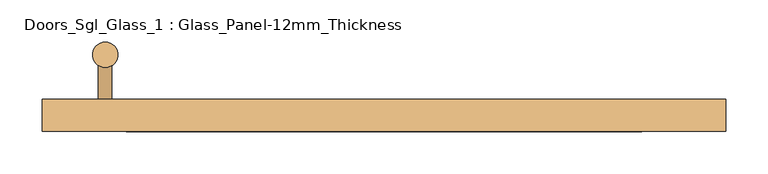
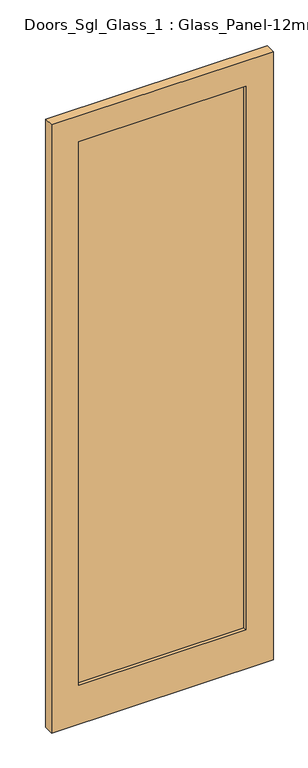
"""IFC4 building model written with IfcOpenShell, lengths in millimetres: door geometry, Doors_Sgl_Glass_1 : Glass_Panel-12mm_Thickness."""

from ifc_helpers import new_model, si_unit, point, frame, frame_2d, origin, place, context, project, spatial, polyline, circle_curve, trimmed, segment, composite_curve, outline, extrude, source, transform, mapped, element, save


def doors_sgl_glass_1_glass_panel_12mm_thickness_d76e1df9(model_context):
    return source(origin(), model_context, "Body", "SweptSolid", [
        extrude(outline(polyline([(306.4578978, 50.0), (306.4578978, 38.0), (-306.4578978, 38.0), (-306.4578978, 50.0), (306.4578978, 50.0)])), frame((0.0, 0.0, 150.0), z_axis=(0.0, 0.0, 1.0), x_axis=(1.0, 0.0, 0.0)), (0.0, 0.0, 1.0), 2105.0),
        extrude(outline(polyline([(0.0, -406.4578978), (0.0, 406.4578978), (2355.0, 406.4578978), (2355.0, -406.4578978), (0.0, -406.4578978)]), holes=[polyline([(2255.0, 306.4578978), (150.0, 306.4578978), (150.0, -306.4578978), (2255.0, -306.4578978), (2255.0, 306.4578978)])]), frame((0.0, 25.0, 0.0), z_axis=(0.0, 1.0, 0.0), x_axis=(0.0, 0.0, 1.0)), (0.0, 0.0, 1.0), 38.0),
        extrude(outline(composite_curve([segment(trimmed(circle_curve(frame_2d((1450.0, -331.4578978)), 8.0), [point((1450.0, -323.4578978))], [point((1450.0, -339.4578978))], False, "CARTESIAN"), True, "CONTINUOUS"), segment(trimmed(circle_curve(frame_2d((1450.0, -331.4578978)), 8.0), [point((1450.0, -339.4578978))], [point((1450.0, -323.4578978))], False, "CARTESIAN"), True, "CONTINUOUS")], self_intersect=False)), frame((0.0, 63.0, 0.0), z_axis=(0.0, 1.0, 0.0), x_axis=(0.0, 0.0, 1.0)), (0.0, 0.0, 1.0), 53.0),
        extrude(outline(composite_curve([segment(trimmed(circle_curve(frame_2d((750.0, -331.4578978)), 8.0), [point((750.0, -323.4578978))], [point((750.0, -339.4578978))], False, "CARTESIAN"), True, "CONTINUOUS"), segment(trimmed(circle_curve(frame_2d((750.0, -331.4578978)), 8.0), [point((750.0, -339.4578978))], [point((750.0, -323.4578978))], False, "CARTESIAN"), True, "CONTINUOUS")], self_intersect=False)), frame((0.0, 63.0, 0.0), z_axis=(0.0, 1.0, 0.0), x_axis=(0.0, 0.0, 1.0)), (0.0, 0.0, 1.0), 53.0),
        extrude(outline(composite_curve([segment(trimmed(circle_curve(frame_2d((-331.4578978, 116.0)), 15.0), [point((-331.4578978, 101.0))], [point((-331.4578978, 131.0))], False, "CARTESIAN"), True, "CONTINUOUS"), segment(trimmed(circle_curve(frame_2d((-331.4578978, 116.0)), 15.0), [point((-331.4578978, 131.0))], [point((-331.4578978, 101.0))], False, "CARTESIAN"), True, "CONTINUOUS")], self_intersect=False)), frame((0.0, 0.0, 650.0), z_axis=(0.0, 0.0, 1.0), x_axis=(1.0, 0.0, 0.0)), (0.0, 0.0, 1.0), 900.0),
    ])


if __name__ == "__main__":
    model = new_model("IFC4")
    model_context = context("Model", 3, world=origin())
    ifc_project = project(units=[si_unit("LENGTHUNIT", "METRE", prefix="MILLI")], contexts=[model_context])
    site = spatial("IfcSite", under=ifc_project)
    building = spatial("IfcBuilding", under=site)
    placement = place(None, origin())
    doors_sgl_glass_1_glass_panel_12mm_thickness_shape = doors_sgl_glass_1_glass_panel_12mm_thickness_d76e1df9(model_context)
    element("IfcDoor", 1, ObjectType="Doors_Sgl_Glass_1 : Glass_Panel-12mm_Thickness", at=placement, inside=building, context=model_context, shape_type="MappedRepresentation", body=[
        mapped(doors_sgl_glass_1_glass_panel_12mm_thickness_shape, transform((0.0, 0.0, 0.0), x_axis=(1.0, 0.0, 0.0), y_axis=(0.0, 1.0, 0.0), z_axis=(0.0, 0.0, 1.0))),
    ])
    save(model, "model.ifc")

# Revit data of these elements
# Type "Doors_Sgl_Glass_1 : Glass_Panel-12mm_Thickness"
#   Type Mark = "60"
#   Construction Type Id = "GSP4R"
#   Keynote = "H11"
#   Analytic Construction = "1/8 in Pilkington single glazing"
#   Visual Light Transmittance = 0.9
#   Stile Top Rail = 0' - 3.93701"
#   Stile Shutting = 0' - 3.93701"
#   Stile Hanging = 0' - 3.93701"
#   Stile Bottom Rail = 0' - 5.90551"
#   Solar Heat Gain Coefficient = 0.78
#   Offset = 0' - 1.9685"
#   Heat Transfer Coefficient (U) = 3.6886 W/(m²·K)
#   Handle X Distance = 0' - 2.95276"
#   Glazing Thickness = 0' - 0.47244"
#   Define Thermal Properties by = 1
#   Material Ironmongery = Metal - Aluminum
#   Material Frame = Metal - Aluminum
#   Material Glass = Glass
#   Function = (empty or 0)
# Element 1 (IfcDoor, "Doors_Sgl_Glass_1 : Glass_Panel-12mm_Thickness")
#   Materials on its faces: "Metal - Aluminum", "Glass"
# Materials
#   "Metal - Aluminum": class "Metal", colour RGB 247 247 247, transparency 0
#   "Glass": class "Glass", colour RGB 0 128 192, transparency 0.9, Description = "Soda Lime Glass", Cost = 0
